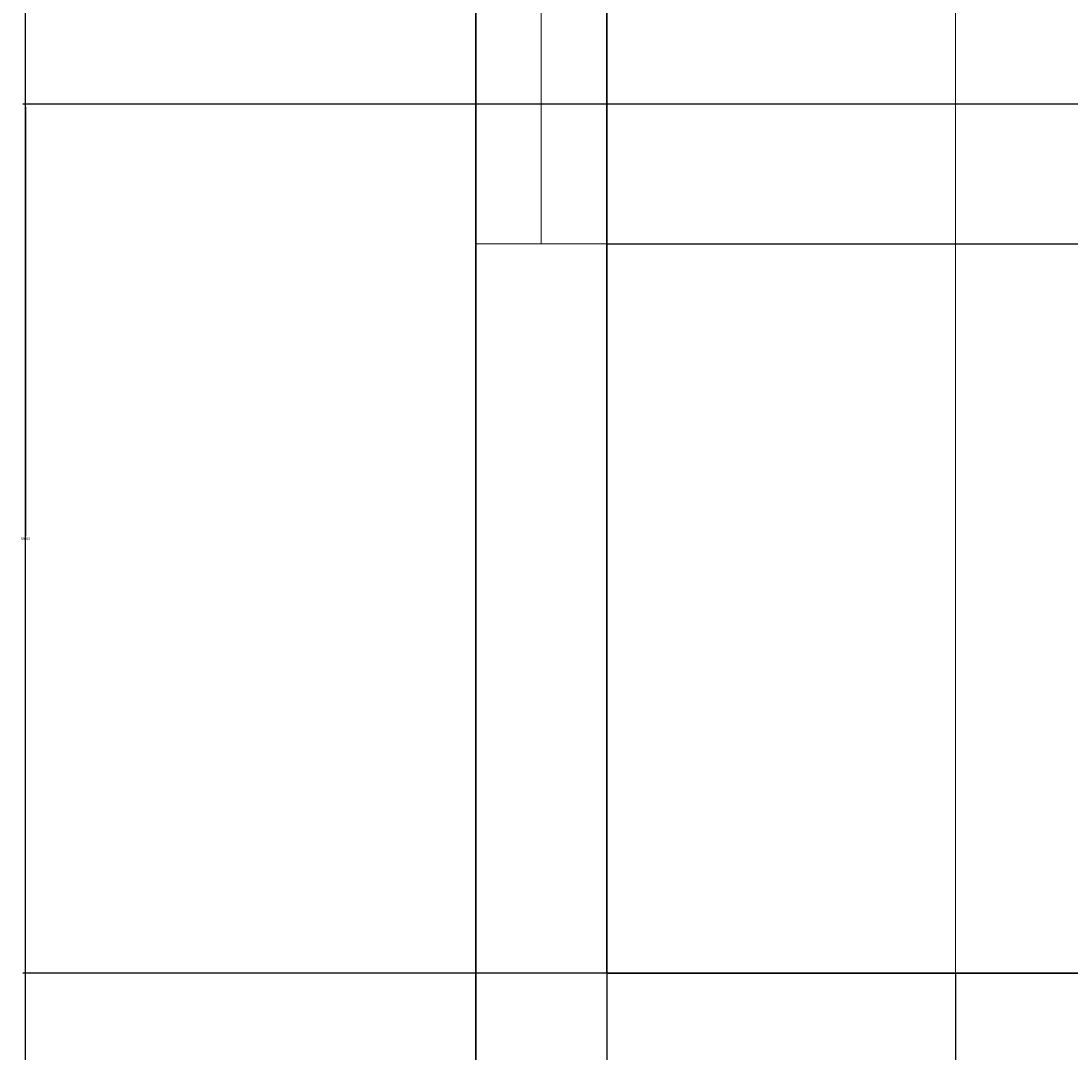
# Model space of a CAD drawing. Units: feet. Extents: x 1654 to 2985, y 1348 to 2230.
# Tile 5 of 53: x 1812 to 1884, y 1746 to 1817. Entities that reach past the tile are written whole.
import ezdxf

# ---------------------------------------------------------------- set-up
doc = ezdxf.new("R2010")
doc.units = ezdxf.units.FT
for name, color, linetype, lineweight in [('A-ANNO-DIMS', 2, 'Continuous', 18), ('A-FLOR-CASE', 8, 'Continuous', 18), ('A-GLAZ', 4, 'Continuous', 18), ('A-WALL', 7, 'Continuous', 35)]:
    doc.layers.add(name, color=color, linetype=linetype, lineweight=lineweight)
doc.styles.get("Standard").update_dxf_attribs({"font": 'arial.ttf'})
doc.dimstyles.get("Standard").update_dxf_attribs({"dimtxt": 0.18, "dimasz": 0.18, "dimexe": 0.18, "dimexo": 0.0625, "dimgap": 0.09, "dimtad": 0, "dimtih": 1, "dimtoh": 1, "dimdec": 4, "dimzin": 0, "dimdsep": 46, "dimtxsty": 'Standard', "dimcen": 0.09, "dimadec": 0, "dimazin": 0, "dimtfac": 1, "dimtdec": 4, "dimtofl": 0, "dimtmove": 0, "dimatfit": 3, "dimfxl": 1, "dimtolj": 1, "dimtzin": 0, "dimarcsym": 0})

# ---------------------------------------------------------------- blocks, each defined once
blk = doc.blocks.new('WIN-KITCHEN')
for p, q in [((0, 60.691), (9, 60.691)), ((4.5, 60.691), (4.5, 0)), ((0, 0), (9, 0))]:
    blk.add_line(p, q)
blk = doc.blocks.new('CASEWORK-KITCHEN-L')
for q in [(72, 111), (0, 0)]:
    blk.add_line((0, 111), q)
blk = doc.blocks.new('*D75')
at = {"layer": 'A-ANNO-DIMS', "color": 0, "lineweight": -2, "transparency": 16777216}
for p, q in [((1876.092, 1751.192), (1876.092, 1734.425)), ((1948.092, 1751.192), (1948.092, 1734.425)), ((1876.272, 1734.605), (1911.565, 1734.605)), ((1947.912, 1734.605), (1912.62, 1734.605))]:
    blk.add_line(p, q, dxfattribs=at)
at = {"layer": 'A-ANNO-DIMS', "color": 0, "transparency": 16777216}
for points in [[(1876.272, 1734.635), (1876.272, 1734.575), (1876.092, 1734.605)], [(1947.912, 1734.635), (1947.912, 1734.575), (1948.092, 1734.605)]]:
    blk.add_solid(points, dxfattribs=at)
at = {"layer": 'Defpoints', "color": 0, "transparency": 16777216}
for p in [(1876.092, 1751.255), (1948.092, 1751.255), (1948.092, 1734.605)]:
    blk.add_point(p, dxfattribs=at)
at = {"layer": 'A-ANNO-DIMS', "color": 0, "transparency": 16777216, "insert": (1912.092, 1734.605), "char_height": 0.18, "attachment_point": 5}
blk.add_mtext('\\A1;72 TYP.', dxfattribs=at)
blk = doc.blocks.new('*D77')
at = {"layer": 'A-ANNO-DIMS', "color": 0, "lineweight": -2, "transparency": 16777216}
for p, q in [((1843.03, 2117.255), (1811.912, 2117.255)), ((1812.092, 2117.075), (1812.092, 1841.437)), ((1812.092, 1565.435), (1812.092, 1841.073)), ((1843.03, 1565.255), (1811.912, 1565.255))]:
    blk.add_line(p, q, dxfattribs=at)
at = {"layer": 'A-ANNO-DIMS', "color": 0, "transparency": 16777216}
for points in [[(1812.062, 2117.075), (1812.122, 2117.075), (1812.092, 2117.255)], [(1812.062, 1565.435), (1812.122, 1565.435), (1812.092, 1565.255)]]:
    blk.add_solid(points, dxfattribs=at)
at = {"layer": 'Defpoints', "color": 0, "transparency": 16777216}
for p in [(1812.092, 2117.255), (1843.092, 2117.255), (1843.092, 1565.255)]:
    blk.add_point(p, dxfattribs=at)
at = {"layer": 'A-ANNO-DIMS', "color": 0, "transparency": 16777216, "insert": (1812.092, 1841.255), "char_height": 0.18, "attachment_point": 5}
blk.add_mtext('\\A1;552', dxfattribs=at)
blk = doc.blocks.new('*D91')
at = {"layer": 'A-ANNO-DIMS', "color": 0, "lineweight": -2, "transparency": 16777216}
for p, q in [((1852.155, 1801.468), (2242.272, 1801.468)), ((2242.092, 1801.288), (2242.092, 1776.544)), ((2242.092, 1751.435), (2242.092, 1776.18)), ((1852.155, 1751.255), (2242.272, 1751.255))]:
    blk.add_line(p, q, dxfattribs=at)
at = {"layer": 'A-ANNO-DIMS', "color": 0, "transparency": 16777216}
for points in [[(2242.062, 1801.288), (2242.122, 1801.288), (2242.092, 1801.468)], [(2242.062, 1751.435), (2242.122, 1751.435), (2242.092, 1751.255)]]:
    blk.add_solid(points, dxfattribs=at)
at = {"layer": 'Defpoints', "color": 0, "transparency": 16777216}
for p in [(1852.092, 1801.468), (2242.092, 1801.468), (1852.092, 1751.255)]:
    blk.add_point(p, dxfattribs=at)
at = {"layer": 'A-ANNO-DIMS', "color": 0, "transparency": 16777216, "insert": (2242.092, 1776.362), "char_height": 0.18, "attachment_point": 5}
blk.add_mtext('\\A1;50.21', dxfattribs=at)
blk = doc.blocks.new('*D98')
at = {"layer": 'A-ANNO-DIMS', "color": 0, "lineweight": -2, "transparency": 16777216}
for p, q in [((2061.03, 1811.081), (1811.912, 1811.081)), ((1812.092, 1810.901), (1812.092, 1781.35)), ((1812.092, 1751.435), (1812.092, 1780.986)), ((2061.03, 1751.255), (1811.912, 1751.255))]:
    blk.add_line(p, q, dxfattribs=at)
at = {"layer": 'A-ANNO-DIMS', "color": 0, "transparency": 16777216}
for points in [[(1812.062, 1810.901), (1812.122, 1810.901), (1812.092, 1811.081)], [(1812.062, 1751.435), (1812.122, 1751.435), (1812.092, 1751.255)]]:
    blk.add_solid(points, dxfattribs=at)
at = {"layer": 'Defpoints', "color": 0, "transparency": 16777216}
for p in [(1812.092, 1811.081), (2061.092, 1811.081), (2061.092, 1751.255)]:
    blk.add_point(p, dxfattribs=at)
at = {"layer": 'A-ANNO-DIMS', "color": 0, "transparency": 16777216, "insert": (1812.092, 1781.168), "char_height": 0.18, "attachment_point": 5}
blk.add_mtext('\\A1;59.83', dxfattribs=at)
blk = doc.blocks.new('*D100')
at = {"layer": 'A-ANNO-DIMS', "color": 0, "lineweight": -2, "transparency": 16777216}
for p, q in [((1852.092, 1751.192), (1852.092, 1534.075)), ((1876.092, 1751.192), (1876.092, 1534.075)), ((1852.272, 1534.255), (1863.872, 1534.255)), ((1875.912, 1534.255), (1864.313, 1534.255))]:
    blk.add_line(p, q, dxfattribs=at)
at = {"layer": 'A-ANNO-DIMS', "color": 0, "transparency": 16777216}
for points in [[(1852.272, 1534.285), (1852.272, 1534.225), (1852.092, 1534.255)], [(1875.912, 1534.285), (1875.912, 1534.225), (1876.092, 1534.255)]]:
    blk.add_solid(points, dxfattribs=at)
at = {"layer": 'Defpoints', "color": 0, "transparency": 16777216}
for p in [(1852.092, 1751.255), (1876.092, 1751.255), (1876.092, 1534.255)]:
    blk.add_point(p, dxfattribs=at)
at = {"layer": 'A-ANNO-DIMS', "color": 0, "transparency": 16777216, "insert": (1864.092, 1534.255), "char_height": 0.18, "attachment_point": 5}
blk.add_mtext('\\A1;24', dxfattribs=at)

msp = doc.modelspace()

# ---------------------------------------------------------------- linework, layer by layer
at = {"layer": 'A-WALL'}
for p, q in [((1843.0924, 2117.2549), (1843.0924, 1565.2549)), ((1843.0924, 1886.2549), (1843.0924, 1751.2549)), ((1852.0924, 1886.2549), (1852.0924, 1751.2549)), ((1852.0924, 1751.2549), (1948.0924, 1751.2549))]:
    msp.add_line(p, q, dxfattribs=at)

# ---------------------------------------------------------------- block references
at = {"layer": 'A-FLOR-CASE'}
msp.add_blockref('CASEWORK-KITCHEN-L', (1876.092, 1751.255), dxfattribs=at)
at = {"layer": 'A-GLAZ'}
msp.add_blockref('WIN-KITCHEN', (1843.092, 1801.468), dxfattribs=at)

# ---------------------------------------------------------------- dimensions: what is measured, and where the dimension line sits
at = {"layer": 'A-ANNO-DIMS'}
for base, p1, p2, override, picture, middle in [((1812.0924, 2117.2549), (1843.0924, 1565.2549), (1843.0924, 2117.2549), {"dimdec": 0, "dimlfac": 1, "dimrnd": 0, "dimzin": 0, "dimdsep": 46, "dimlunit": 2}, '*D77', (1812.0924, 1841.2549)), ((1812.0924, 1811.0815), (2061.0924, 1751.2549), (2061.0924, 1811.0815), {"dimdec": 2, "dimlfac": 1, "dimrnd": 0, "dimzin": 0, "dimdsep": 46, "dimlunit": 2}, '*D98', (1812.0924, 1781.1682)), ((2242.0924, 1801.4683), (1852.0924, 1751.2549), (1852.0924, 1801.4683), {"dimdec": 2, "dimlfac": 1, "dimrnd": 0, "dimzin": 0, "dimdsep": 46, "dimlunit": 2}, '*D91', (2242.0924, 1776.3616))]:
    dim = msp.add_linear_dim(base=base, p1=p1, p2=p2, angle=90, dimstyle='Standard', override=override, dxfattribs=at)
    dim.commit()
    dim.dimension.update_dxf_attribs({"geometry": picture, "text_midpoint": middle})
dim = msp.add_linear_dim(base=(1876.0924, 1534.2549), p1=(1852.0924, 1751.2549), p2=(1876.0924, 1751.2549), dimstyle='Standard', override={"dimdec": 0, "dimlfac": 1, "dimrnd": 0, "dimzin": 0, "dimdsep": 46, "dimlunit": 2}, dxfattribs=at)
dim.commit()
dim.dimension.update_dxf_attribs({"geometry": '*D100', "text_midpoint": (1864.0924, 1534.2549)})
dim = msp.add_linear_dim(base=(1948.0924, 1734.6049), p1=(1876.0924, 1751.2549), p2=(1948.0924, 1751.2549), text='<> TYP.', dimstyle='Standard', override={"dimdec": 0, "dimlfac": 1, "dimrnd": 0, "dimzin": 0, "dimdsep": 46, "dimlunit": 2}, dxfattribs=at)
dim.commit()
dim.dimension.update_dxf_attribs({"geometry": '*D75', "text_midpoint": (1912.0924, 1734.6049)})

doc.saveas('drawing.dxf')
